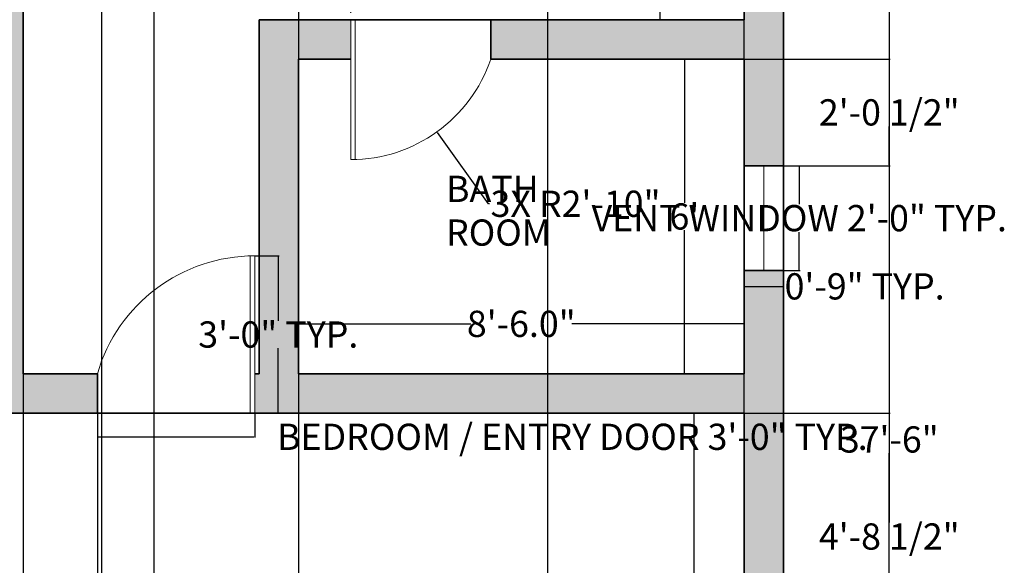
# Model space of a CAD drawing. Units: inches. Extents: x 1174 to 1615, y 3112 to 3628.
# Tile 5 of 6: x 1390 to 1615, y 3341 to 3466. Entities that reach past the tile are written whole.
import ezdxf

# ---------------------------------------------------------------- set-up
doc = ezdxf.new("R2010")
doc.units = ezdxf.units.IN
doc.header["$MEASUREMENT"] = 0
doc.layers.get('0').update_dxf_attribs({"color": 250})
for name, color, linetype, lineweight in [('A-ANNO-DIMS', 2, 'Continuous', 18), ('A-AREA-IDEN', 7, 'Continuous', 25), ('A-DOOR', 3, 'Continuous', 18), ('A-GLAZ', 4, 'Continuous', 18), ('A-WALL', 7, 'Continuous', 35)]:
    doc.layers.add(name, color=color, linetype=linetype, lineweight=lineweight)
doc.layers.add('A-WALL-PATT', color=18, linetype='Continuous', lineweight=13, true_color=0x000000)
doc.styles.get("Standard").update_dxf_attribs({"font": 'arial.ttf'})
doc.dimstyles.get("Standard").update_dxf_attribs({"dimtxt": 6, "dimasz": 0.18, "dimexe": 0.18, "dimexo": 0.0625, "dimgap": 0.09, "dimtad": 0, "dimtih": 1, "dimtoh": 1, "dimdec": 1, "dimzin": 0, "dimdsep": 46, "dimlunit": 3, "dimtxsty": 'Standard', "dimcen": 0.09, "dimadec": 0, "dimazin": 0, "dimtfac": 1, "dimtdec": 1, "dimtofl": 0, "dimtmove": 0, "dimatfit": 3, "dimfxl": 1, "dimtolj": 1, "dimtzin": 0, "dimarcsym": 0})

# ---------------------------------------------------------------- blocks, each defined once
blk = doc.blocks.new('*D9')
at = {"layer": 'A-ANNO-DIMS', "color": 0, "lineweight": -2, "transparency": 16777216}
for p, q in [((1453.66, 3385.09), (1453.66, 3396.65)), ((1453.84, 3396.47), (1493.1, 3396.47)), ((1555.48, 3396.47), (1516.23, 3396.47)), ((1555.66, 3385.09), (1555.66, 3396.65))]:
    blk.add_line(p, q, dxfattribs=at)
at = {"layer": 'A-ANNO-DIMS', "color": 0, "transparency": 16777216}
for points in [[(1453.84, 3396.5), (1453.84, 3396.44), (1453.66, 3396.47)], [(1555.48, 3396.5), (1555.48, 3396.44), (1555.66, 3396.47)]]:
    blk.add_solid(points, dxfattribs=at)
at = {"layer": 'Defpoints', "color": 0, "transparency": 16777216}
for p in [(1555.66, 3396.47), (1453.66, 3385.03), (1555.66, 3385.03)]:
    blk.add_point(p, dxfattribs=at)
at = {"layer": 'A-ANNO-DIMS', "color": 0, "transparency": 16777216, "insert": (1504.66, 3396.47), "char_height": 6, "attachment_point": 5}
blk.add_mtext('\\A1;8\'-6.0"', dxfattribs=at)
blk = doc.blocks.new('*D10')
at = {"layer": 'A-ANNO-DIMS', "color": 0, "lineweight": -2, "transparency": 16777216}
for p, q in [((1555.6, 3457.03), (1541.81, 3457.03)), ((1541.99, 3456.85), (1541.99, 3424.18)), ((1541.99, 3385.21), (1541.99, 3417.88)), ((1555.6, 3385.03), (1541.81, 3385.03))]:
    blk.add_line(p, q, dxfattribs=at)
at = {"layer": 'A-ANNO-DIMS', "color": 0, "transparency": 16777216}
for points in [[(1541.96, 3456.85), (1542.02, 3456.85), (1541.99, 3457.03)], [(1541.96, 3385.21), (1542.02, 3385.21), (1541.99, 3385.03)]]:
    blk.add_solid(points, dxfattribs=at)
at = {"layer": 'Defpoints', "color": 0, "transparency": 16777216}
for p in [(1555.66, 3457.03), (1541.99, 3385.03), (1555.66, 3385.03)]:
    blk.add_point(p, dxfattribs=at)
at = {"layer": 'A-ANNO-DIMS', "color": 0, "transparency": 16777216, "insert": (1541.99, 3421.03), "char_height": 6, "attachment_point": 5}
blk.add_mtext("\\A1;6'", dxfattribs=at)
blk = doc.blocks.new('*D12')
at = {"layer": 'A-ANNO-DIMS', "color": 0, "lineweight": -2, "transparency": 16777216}
for p, q in [((1555.6, 3376.03), (1544, 3376.03)), ((1544.18, 3375.85), (1544.18, 3283.18)), ((1544.18, 3184.21), (1544.18, 3276.88)), ((1555.6, 3184.03), (1544, 3184.03))]:
    blk.add_line(p, q, dxfattribs=at)
at = {"layer": 'A-ANNO-DIMS', "color": 0, "transparency": 16777216}
for points in [[(1544.15, 3375.85), (1544.21, 3375.85), (1544.18, 3376.03)], [(1544.15, 3184.21), (1544.21, 3184.21), (1544.18, 3184.03)]]:
    blk.add_solid(points, dxfattribs=at)
at = {"layer": 'Defpoints', "color": 0, "transparency": 16777216}
for p in [(1555.66, 3376.03), (1544.18, 3184.03), (1555.66, 3184.03)]:
    blk.add_point(p, dxfattribs=at)
at = {"layer": 'A-ANNO-DIMS', "color": 0, "transparency": 16777216, "insert": (1544.18, 3280.03), "char_height": 6, "attachment_point": 5}
blk.add_mtext("\\A1;16'", dxfattribs=at)
blk = doc.blocks.new('*D15')
at = {"layer": 'A-ANNO-DIMS', "color": 0, "lineweight": -2, "transparency": 16777216}
for p, q in [((1555.6, 3586.03), (1536.24, 3586.03)), ((1536.42, 3585.85), (1536.42, 3529.18)), ((1536.42, 3466.21), (1536.42, 3522.88)), ((1555.6, 3466.03), (1536.24, 3466.03))]:
    blk.add_line(p, q, dxfattribs=at)
at = {"layer": 'A-ANNO-DIMS', "color": 0, "transparency": 16777216}
for points in [[(1536.39, 3585.85), (1536.45, 3585.85), (1536.42, 3586.03)], [(1536.39, 3466.21), (1536.45, 3466.21), (1536.42, 3466.03)]]:
    blk.add_solid(points, dxfattribs=at)
at = {"layer": 'Defpoints', "color": 0, "transparency": 16777216}
for p in [(1555.66, 3586.03), (1536.42, 3466.03), (1555.66, 3466.03)]:
    blk.add_point(p, dxfattribs=at)
at = {"layer": 'A-ANNO-DIMS', "color": 0, "transparency": 16777216, "insert": (1536.42, 3526.03), "char_height": 6, "attachment_point": 5}
blk.add_mtext("\\A1;10'", dxfattribs=at)
blk = doc.blocks.new('DOOR-SWING-36IN')
for p, q in [((-1, 36), (-1, 0)), ((0, 0), (0, 36)), ((0, 0), (-36, 0))]:
    blk.add_line(p, q)
blk.add_arc((0, -1.5), 37.5, 90, 163.7398)
blk = doc.blocks.new('DOOR-SWING-32IN')
for p, q in [((0, 0), (0, -32)), ((0, 0), (32, 0)), ((1, -32), (1, 0))]:
    blk.add_line(p, q)
blk.add_arc((0, 1.76), 33.76, 270, 341.4134)
blk = doc.blocks.new('VENT-WINDOW-24IN')
for p, q in [((-4.5, -24), (-4.5, 0)), ((0, 0), (0, -24)), ((4.5, 0), (4.5, -24))]:
    blk.add_line(p, q)
blk = doc.blocks.new('*D28')
at = {"layer": 'A-ANNO-DIMS', "color": 0, "lineweight": -2, "transparency": 16777216}
for p, q in [((1564.73, 3432.64), (1568.44, 3432.64)), ((1568.26, 3432.46), (1568.26, 3423.83)), ((1568.26, 3408.82), (1568.26, 3417.44)), ((1564.73, 3408.64), (1568.44, 3408.64))]:
    blk.add_line(p, q, dxfattribs=at)
at = {"layer": 'A-ANNO-DIMS', "color": 0, "transparency": 16777216}
for points in [[(1568.23, 3432.46), (1568.29, 3432.46), (1568.26, 3432.64)], [(1568.23, 3408.82), (1568.29, 3408.82), (1568.26, 3408.64)]]:
    blk.add_solid(points, dxfattribs=at)
at = {"layer": 'Defpoints', "color": 0, "transparency": 16777216}
for p in [(1564.66, 3432.64), (1568.26, 3432.64), (1564.66, 3408.64)]:
    blk.add_point(p, dxfattribs=at)
at = {"layer": 'A-ANNO-DIMS', "color": 0, "transparency": 16777216, "insert": (1568.26, 3420.64), "char_height": 6, "attachment_point": 5}
blk.add_mtext('\\A1;VENT WINDOW 2\'-0" TYP.', dxfattribs=at)
blk = doc.blocks.new('*D29')
at = {"layer": 'A-ANNO-DIMS', "color": 0, "lineweight": -2, "transparency": 16777216}
for p, q in [((1555.66, 3408.58), (1555.66, 3404.86)), ((1564.66, 3408.58), (1564.66, 3404.86)), ((1555.84, 3405.04), (1564.48, 3405.04)), ((1564.66, 3405.04), (1564.84, 3405.04))]:
    blk.add_line(p, q, dxfattribs=at)
at = {"layer": 'A-ANNO-DIMS', "color": 0, "transparency": 16777216}
for points in [[(1555.84, 3405.07), (1555.84, 3405.01), (1555.66, 3405.04)], [(1564.48, 3405.07), (1564.48, 3405.01), (1564.66, 3405.04)]]:
    blk.add_solid(points, dxfattribs=at)
at = {"layer": 'Defpoints', "color": 0, "transparency": 16777216}
for p in [(1555.66, 3408.64), (1564.66, 3408.64), (1564.66, 3405.04)]:
    blk.add_point(p, dxfattribs=at)
at = {"layer": 'A-ANNO-DIMS', "color": 0, "transparency": 16777216, "insert": (1583.22, 3405.04), "char_height": 6, "attachment_point": 5}
blk.add_mtext('\\A1;0\'-9" TYP.', dxfattribs=at)
blk = doc.blocks.new('*D36')
at = {"layer": 'A-ANNO-DIMS', "color": 0, "lineweight": -2, "transparency": 16777216}
for p, q in [((1407.66, 3375.97), (1407.66, 3370.45)), ((1443.66, 3375.97), (1443.66, 3370.45)), ((1407.84, 3370.63), (1443.48, 3370.63)), ((1443.66, 3370.63), (1443.84, 3370.63))]:
    blk.add_line(p, q, dxfattribs=at)
at = {"layer": 'A-ANNO-DIMS', "color": 0, "transparency": 16777216}
for points in [[(1407.84, 3370.66), (1407.84, 3370.6), (1407.66, 3370.63)], [(1443.48, 3370.66), (1443.48, 3370.6), (1443.66, 3370.63)]]:
    blk.add_solid(points, dxfattribs=at)
at = {"layer": 'Defpoints', "color": 0, "transparency": 16777216}
for p in [(1407.66, 3376.03), (1443.66, 3376.03), (1443.66, 3370.63)]:
    blk.add_point(p, dxfattribs=at)
at = {"layer": 'A-ANNO-DIMS', "color": 0, "transparency": 16777216, "insert": (1516.34, 3370.63), "char_height": 6, "attachment_point": 5}
blk.add_mtext('\\A1;BEDROOM / ENTRY DOOR 3\'-0" TYP.', dxfattribs=at)
blk = doc.blocks.new('*D37')
at = {"layer": 'A-ANNO-DIMS', "color": 0, "lineweight": -2, "transparency": 16777216}
for p, q in [((1443.73, 3412.03), (1449.24, 3412.03)), ((1449.06, 3411.85), (1449.06, 3397.18)), ((1449.06, 3376.21), (1449.06, 3390.87)), ((1443.73, 3376.03), (1449.24, 3376.03))]:
    blk.add_line(p, q, dxfattribs=at)
at = {"layer": 'A-ANNO-DIMS', "color": 0, "transparency": 16777216}
for points in [[(1449.03, 3411.85), (1449.09, 3411.85), (1449.06, 3412.03)], [(1449.03, 3376.21), (1449.09, 3376.21), (1449.06, 3376.03)]]:
    blk.add_solid(points, dxfattribs=at)
at = {"layer": 'Defpoints', "color": 0, "transparency": 16777216}
for p in [(1443.66, 3412.03), (1449.06, 3412.03), (1443.66, 3376.03)]:
    blk.add_point(p, dxfattribs=at)
at = {"layer": 'A-ANNO-DIMS', "color": 0, "transparency": 16777216, "insert": (1449.06, 3394.03), "char_height": 6, "attachment_point": 5}
blk.add_mtext('\\A1;3\'-0" TYP.', dxfattribs=at)
blk = doc.blocks.new('*D41')
at = {"layer": 'A-ANNO-DIMS', "color": 0, "lineweight": -2, "transparency": 16777216}
for p, q in [((1564.73, 3595.03), (1589.04, 3595.03)), ((1588.86, 3594.85), (1588.86, 3373.18)), ((1588.86, 3145.21), (1588.86, 3366.87)), ((1439.51, 3145.03), (1589.04, 3145.03))]:
    blk.add_line(p, q, dxfattribs=at)
at = {"layer": 'A-ANNO-DIMS', "color": 0, "transparency": 16777216}
for points in [[(1588.83, 3594.85), (1588.89, 3594.85), (1588.86, 3595.03)], [(1588.83, 3145.21), (1588.89, 3145.21), (1588.86, 3145.03)]]:
    blk.add_solid(points, dxfattribs=at)
at = {"layer": 'Defpoints', "color": 0, "transparency": 16777216}
for p in [(1564.66, 3595.03), (1588.86, 3595.03), (1439.45, 3145.03)]:
    blk.add_point(p, dxfattribs=at)
at = {"layer": 'A-ANNO-DIMS', "color": 0, "transparency": 16777216, "insert": (1588.86, 3370.03), "char_height": 6, "attachment_point": 5}
blk.add_mtext('\\A1;37\'-6"', dxfattribs=at)
blk = doc.blocks.new('*D49')
at = {"layer": 'A-ANNO-DIMS', "color": 0, "lineweight": -2, "transparency": 16777216}
for p, q in [((1225.73, 3376.03), (1589.04, 3376.03)), ((1588.86, 3375.85), (1588.86, 3351.02)), ((1588.86, 3319.81), (1588.86, 3344.64)), ((1225.73, 3319.63), (1589.04, 3319.63))]:
    blk.add_line(p, q, dxfattribs=at)
at = {"layer": 'A-ANNO-DIMS', "color": 0, "transparency": 16777216}
for points in [[(1588.83, 3375.85), (1588.89, 3375.85), (1588.86, 3376.03)], [(1588.83, 3319.81), (1588.89, 3319.81), (1588.86, 3319.63)]]:
    blk.add_solid(points, dxfattribs=at)
at = {"layer": 'Defpoints', "color": 0, "transparency": 16777216}
for p in [(1225.66, 3376.03), (1225.66, 3319.63), (1588.86, 3319.63)]:
    blk.add_point(p, dxfattribs=at)
at = {"layer": 'A-ANNO-DIMS', "color": 0, "transparency": 16777216, "insert": (1588.86, 3347.83), "char_height": 6, "attachment_point": 5}
blk.add_mtext('\\A1;4\'-8 1/2"', dxfattribs=at)
blk = doc.blocks.new('*D51')
at = {"layer": 'A-ANNO-DIMS', "color": 0, "lineweight": -2, "transparency": 16777216}
for p, q in [((1555.73, 3457.03), (1589.04, 3457.03)), ((1588.86, 3456.85), (1588.86, 3448.03)), ((1588.86, 3432.82), (1588.86, 3441.64)), ((1564.73, 3432.64), (1589.04, 3432.64))]:
    blk.add_line(p, q, dxfattribs=at)
at = {"layer": 'A-ANNO-DIMS', "color": 0, "transparency": 16777216}
for points in [[(1588.83, 3456.85), (1588.89, 3456.85), (1588.86, 3457.03)], [(1588.83, 3432.82), (1588.89, 3432.82), (1588.86, 3432.64)]]:
    blk.add_solid(points, dxfattribs=at)
at = {"layer": 'Defpoints', "color": 0, "transparency": 16777216}
for p in [(1555.66, 3457.03), (1588.86, 3457.03), (1564.66, 3432.64)]:
    blk.add_point(p, dxfattribs=at)
at = {"layer": 'A-ANNO-DIMS', "color": 0, "transparency": 16777216, "insert": (1588.86, 3444.83), "char_height": 6, "attachment_point": 5}
blk.add_mtext('\\A1;2\'-0 1/2"', dxfattribs=at)
blk = doc.blocks.new('*D52')
at = {"layer": 'A-ANNO-DIMS', "color": 0, "lineweight": -2, "transparency": 16777216}
for p, q in [((1555.6, 3376.03), (1192.28, 3376.03)), ((1192.46, 3375.85), (1192.46, 3351.26)), ((1192.46, 3320.35), (1192.46, 3344.95)), ((1555.6, 3320.17), (1192.28, 3320.17))]:
    blk.add_line(p, q, dxfattribs=at)
at = {"layer": 'A-ANNO-DIMS', "color": 0, "transparency": 16777216}
for points in [[(1192.43, 3375.85), (1192.49, 3375.85), (1192.46, 3376.03)], [(1192.43, 3320.35), (1192.49, 3320.35), (1192.46, 3320.17)]]:
    blk.add_solid(points, dxfattribs=at)
at = {"layer": 'Defpoints', "color": 0, "transparency": 16777216}
for p in [(1555.66, 3376.03), (1192.46, 3320.17), (1555.66, 3320.17)]:
    blk.add_point(p, dxfattribs=at)
at = {"layer": 'A-ANNO-DIMS', "color": 0, "transparency": 16777216, "insert": (1192.46, 3348.1), "char_height": 6, "attachment_point": 5}
blk.add_mtext('\\A1;4\'-8"', dxfattribs=at)
blk = doc.blocks.new('*D57')
at = {"layer": 'A-ANNO-DIMS', "color": 0, "lineweight": -2, "transparency": 16777216}
for p, q in [((1390.66, 3384.97), (1390.66, 3120.65)), ((1407.66, 3384.97), (1407.66, 3120.65)), ((1390.84, 3120.83), (1391.38, 3120.83)), ((1407.48, 3120.83), (1406.95, 3120.83))]:
    blk.add_line(p, q, dxfattribs=at)
at = {"layer": 'A-ANNO-DIMS', "color": 0, "transparency": 16777216}
for points in [[(1390.84, 3120.86), (1390.84, 3120.8), (1390.66, 3120.83)], [(1407.48, 3120.86), (1407.48, 3120.8), (1407.66, 3120.83)]]:
    blk.add_solid(points, dxfattribs=at)
at = {"layer": 'Defpoints', "color": 0, "transparency": 16777216}
for p in [(1390.66, 3385.03), (1407.66, 3385.03), (1407.66, 3120.83)]:
    blk.add_point(p, dxfattribs=at)
at = {"layer": 'A-ANNO-DIMS', "color": 0, "transparency": 16777216, "insert": (1399.16, 3120.83), "char_height": 6, "attachment_point": 5}
blk.add_mtext('\\A1;1\'-5"', dxfattribs=at)
blk = doc.blocks.new('*D59')
at = {"layer": 'A-ANNO-DIMS', "color": 0, "lineweight": -2, "transparency": 16777216}
for p, q in [((1408.66, 3268.09), (1408.66, 3619.41)), ((1408.84, 3619.23), (1420.48, 3619.23)), ((1420.66, 3268.09), (1420.66, 3619.41)), ((1420.66, 3619.23), (1420.84, 3619.23))]:
    blk.add_line(p, q, dxfattribs=at)
at = {"layer": 'A-ANNO-DIMS', "color": 0, "transparency": 16777216}
for points in [[(1408.84, 3619.26), (1408.84, 3619.2), (1408.66, 3619.23)], [(1420.48, 3619.26), (1420.48, 3619.2), (1420.66, 3619.23)]]:
    blk.add_solid(points, dxfattribs=at)
at = {"layer": 'Defpoints', "color": 0, "transparency": 16777216}
for p in [(1420.66, 3619.23), (1408.66, 3268.03), (1420.66, 3268.03)]:
    blk.add_point(p, dxfattribs=at)
at = {"layer": 'A-ANNO-DIMS', "color": 0, "transparency": 16777216, "insert": (1428.63, 3619.23), "char_height": 6, "attachment_point": 5}
blk.add_mtext('\\A1;1\'-0"', dxfattribs=at)
blk = doc.blocks.new('*D70')
at = {"layer": 'A-ANNO-DIMS', "color": 0, "lineweight": -2, "transparency": 16777216}
for p, q in [((1390.66, 3585.97), (1390.66, 3120.65)), ((1453.68, 3583.03), (1453.68, 3120.65)), ((1390.84, 3120.83), (1414.11, 3120.83)), ((1453.5, 3120.83), (1430.24, 3120.83))]:
    blk.add_line(p, q, dxfattribs=at)
at = {"layer": 'A-ANNO-DIMS', "color": 0, "transparency": 16777216}
for points in [[(1390.84, 3120.86), (1390.84, 3120.8), (1390.66, 3120.83)], [(1453.5, 3120.86), (1453.5, 3120.8), (1453.68, 3120.83)]]:
    blk.add_solid(points, dxfattribs=at)
at = {"layer": 'Defpoints', "color": 0, "transparency": 16777216}
for p in [(1390.66, 3586.03), (1453.68, 3583.1), (1453.68, 3120.83)]:
    blk.add_point(p, dxfattribs=at)
at = {"layer": 'A-ANNO-DIMS', "color": 0, "transparency": 16777216, "insert": (1422.17, 3120.83), "char_height": 6, "attachment_point": 5}
blk.add_mtext('\\A1;5\'-3"', dxfattribs=at)
blk = doc.blocks.new('*D73')
at = {"layer": 'A-ANNO-DIMS', "color": 0, "lineweight": -2, "transparency": 16777216}
for p, q in [((1510.72, 3286.5), (1510.72, 3619.41)), ((1510.9, 3619.23), (1525.13, 3619.23)), ((1555.48, 3619.23), (1541.25, 3619.23)), ((1555.66, 3284.24), (1555.66, 3619.41))]:
    blk.add_line(p, q, dxfattribs=at)
at = {"layer": 'A-ANNO-DIMS', "color": 0, "transparency": 16777216}
for points in [[(1510.9, 3619.26), (1510.9, 3619.2), (1510.72, 3619.23)], [(1555.48, 3619.26), (1555.48, 3619.2), (1555.66, 3619.23)]]:
    blk.add_solid(points, dxfattribs=at)
at = {"layer": 'Defpoints', "color": 0, "transparency": 16777216}
for p in [(1510.72, 3619.23), (1510.72, 3286.44), (1555.66, 3284.17)]:
    blk.add_point(p, dxfattribs=at)
at = {"layer": 'A-ANNO-DIMS', "color": 0, "transparency": 16777216, "insert": (1533.19, 3619.23), "char_height": 6, "attachment_point": 5}
blk.add_mtext('\\A1;3\'-9"', dxfattribs=at)
blk = doc.blocks.new('*D77')
at = {"layer": 'A-ANNO-DIMS', "color": 0, "lineweight": -2, "transparency": 16777216}
for p, q in [((1465.57, 3467.79), (1465.75, 3467.79)), ((1465.66, 3467.7), (1465.66, 3467.88)), ((1497.19, 3423.93), (1485.47, 3440.23)), ((1497.37, 3423.93), (1497.19, 3423.93))]:
    blk.add_line(p, q, dxfattribs=at)
at = {"layer": 'A-ANNO-DIMS', "color": 0, "transparency": 16777216}
blk.add_solid([(1485.5, 3440.25), (1485.45, 3440.21), (1485.37, 3440.38)], dxfattribs=at)
at = {"layer": 'Defpoints', "color": 0, "transparency": 16777216}
for p in [(1465.66, 3467.79), (1485.37, 3440.38)]:
    blk.add_point(p, dxfattribs=at)
at = {"layer": 'A-ANNO-DIMS', "color": 0, "transparency": 16777216, "insert": (1517.08, 3423.93), "char_height": 6, "attachment_point": 5}
blk.add_mtext('\\A1;3X R2\'-10"', dxfattribs=at)

msp = doc.modelspace()

# ---------------------------------------------------------------- hatches: boundary and pattern name
at = {"layer": 'A-WALL-PATT'}
h = msp.add_hatch(color=256, dxfattribs=at)
h.dxf.hatch_style = 1
h.paths.add_polyline_path([(1564.66, 3595.03), (1216.66, 3595.03), (1216.66, 3564.55), (1225.66, 3564.55), (1225.66, 3586.03), (1381.66, 3586.03), (1381.66, 3385.03), (1380.66, 3385.03), (1380.66, 3376.03), (1381.66, 3376.03), (1407.66, 3376.03), (1407.66, 3385.03), (1390.66, 3385.03), (1390.66, 3586.03), (1555.66, 3586.03), (1555.66, 3558.83), (1564.66, 3558.83)])
h.paths.add_polyline_path([(1564.66, 3408.64), (1555.66, 3408.64), (1555.66, 3385.03), (1453.66, 3385.03), (1453.66, 3457.03), (1465.66, 3457.03), (1465.66, 3466.03), (1453.66, 3466.03), (1444.66, 3466.03), (1444.66, 3385.03), (1443.66, 3385.03), (1443.66, 3376.03), (1444.66, 3376.03), (1555.66, 3376.03), (1555.66, 3320.17), (1564.66, 3320.17)])
h.paths.add_polyline_path([(1564.66, 3522.83), (1555.66, 3522.83), (1555.66, 3466.03), (1497.66, 3466.03), (1497.66, 3457.03), (1555.66, 3457.03), (1555.66, 3432.64), (1564.66, 3432.64)], flags=17)
h.paths.add_polyline_path([(1344.66, 3385.03), (1336.66, 3385.03), (1336.66, 3466.03), (1269.66, 3466.03), (1269.66, 3457.03), (1327.66, 3457.03), (1327.66, 3385.03), (1225.66, 3385.03), (1225.66, 3413.31), (1216.66, 3413.31), (1216.66, 3319.63), (1225.66, 3319.63), (1225.66, 3376.03), (1344.66, 3376.03)])
h.paths.add_polyline_path([(1237.66, 3466.03), (1225.66, 3466.03), (1225.66, 3528.55), (1216.66, 3528.55), (1216.66, 3437.31), (1225.66, 3437.31), (1225.66, 3457.03), (1237.66, 3457.03)], flags=17)
h.paths.add_polyline_path([(1265.25, 3184.03), (1225.66, 3184.03), (1225.66, 3283.63), (1216.66, 3283.63), (1216.66, 3175.03), (1265.25, 3175.03)])
h.paths.add_polyline_path([(1372.66, 3184.03), (1360.66, 3184.03), (1360.66, 3268.03), (1376.66, 3268.03), (1376.66, 3277.03), (1360.66, 3277.03), (1360.66, 3313.03), (1351.66, 3313.03), (1351.66, 3184.03), (1301.25, 3184.03), (1301.25, 3175.03), (1372.66, 3175.03)])
h.paths.add_polyline_path([(1460.02, 3184.03), (1429.66, 3184.03), (1429.66, 3277.03), (1408.66, 3277.03), (1408.66, 3268.03), (1420.66, 3268.03), (1420.66, 3184.03), (1408.66, 3184.03), (1408.66, 3175.03), (1460.02, 3175.03)])
h.paths.add_polyline_path([(1564.66, 3284.17), (1555.66, 3284.17), (1555.66, 3184.03), (1520.02, 3184.03), (1520.02, 3175.03), (1564.66, 3175.03)])

# ---------------------------------------------------------------- linework, layer by layer
at = {"layer": 'A-DOOR'}
for p, q in [((1465.66, 3434.03), (1465.66, 3466.03)), ((1443.66, 3412.03), (1443.66, 3376.03))]:
    msp.add_line(p, q, dxfattribs=at)
at = {"layer": 'A-WALL'}
for p, q in [((1564.66, 3595.03), (1564.66, 3175.03)), ((1390.66, 3586.03), (1390.66, 3385.03)), ((1555.66, 3586.03), (1555.66, 3466.03)), ((1444.66, 3466.03), (1444.66, 3385.03)), ((1444.66, 3466.03), (1555.66, 3466.03)), ((1453.66, 3466.03), (1465.66, 3466.03)), ((1497.66, 3466.03), (1497.66, 3457.03)), ((1453.66, 3457.03), (1453.66, 3385.03)), ((1453.66, 3457.03), (1465.66, 3457.03)), ((1497.66, 3457.03), (1555.66, 3457.03)), ((1555.66, 3457.03), (1555.66, 3385.03)), ((1555.66, 3432.64), (1564.66, 3432.64)), ((1564.66, 3408.64), (1555.66, 3408.64)), ((1390.66, 3385.03), (1407.66, 3385.03)), ((1407.66, 3376.03), (1407.66, 3385.03)), ((1443.66, 3385.03), (1444.66, 3385.03)), ((1453.66, 3385.03), (1555.66, 3385.03)), ((1225.66, 3376.03), (1555.66, 3376.03)), ((1444.66, 3376.03), (1443.66, 3376.03)), ((1555.66, 3376.03), (1555.66, 3184.03))]:
    msp.add_line(p, q, dxfattribs=at)

# ---------------------------------------------------------------- block references
at = {"layer": 'A-DOOR'}
for name, p in [('DOOR-SWING-32IN', (1465.66, 3466.03)), ('DOOR-SWING-36IN', (1443.66, 3376.03))]:
    msp.add_blockref(name, p, dxfattribs=at)
at = {"layer": 'A-GLAZ'}
msp.add_blockref('VENT-WINDOW-24IN', (1560.16, 3432.64), dxfattribs=at)

# ---------------------------------------------------------------- texts
at = {"layer": 'A-AREA-IDEN', "insert": (1487.44, 3430.34), "char_height": 6, "attachment_point": 1}
msp.add_mtext_dynamic_manual_height_columns('BATH\\PROOM', width=57.8599, gutter_width=1, heights=[0], dxfattribs=at)

# ---------------------------------------------------------------- dimensions: what is measured, and where the dimension line sits
at = {"layer": 'A-ANNO-DIMS'}
for base, p1, p2, override, picture, middle in [((1420.66, 3619.23), (1408.66, 3268.03), (1420.66, 3268.03), {"dimdec": 1, "dimlfac": 1, "dimrnd": 0, "dimzin": 1, "dimdsep": 46, "dimlunit": 4, "dimfrac": 2}, '*D59', (1428.63, 3619.23)), ((1510.72, 3619.23), (1555.66, 3284.17), (1510.72, 3286.44), {"dimdec": 1, "dimlfac": 1, "dimrnd": 0, "dimzin": 1, "dimdsep": 46, "dimlunit": 4, "dimfrac": 2}, '*D73', (1533.19, 3619.23)), ((1453.68, 3120.83), (1390.66, 3586.03), (1453.68, 3583.1), {"dimdec": 1, "dimlfac": 1, "dimrnd": 0, "dimzin": 1, "dimdsep": 46, "dimlunit": 4, "dimfrac": 2}, '*D70', (1422.17, 3120.83)), ((1555.66, 3396.47), (1453.66, 3385.03), (1555.66, 3385.03), {"dimclrd": 0, "dimclre": 0, "dimclrt": 0}, '*D9', (1504.66, 3396.47)), ((1407.66, 3120.83), (1390.66, 3385.03), (1407.66, 3385.03), {"dimdec": 1, "dimlfac": 1, "dimrnd": 0, "dimzin": 1, "dimdsep": 46, "dimlunit": 4, "dimfrac": 2}, '*D57', (1399.16, 3120.83))]:
    dim = msp.add_linear_dim(base=base, p1=p1, p2=p2, dimstyle='Standard', override=override, dxfattribs=at)
    dim.commit()
    dim.dimension.update_dxf_attribs({"geometry": picture, "text_midpoint": middle})
for base, p1, p2, override, picture, middle in [((1588.86, 3595.03), (1439.45, 3145.03), (1564.66, 3595.03), {"dimdec": 1, "dimlfac": 1, "dimrnd": 0, "dimzin": 1, "dimdsep": 46, "dimlunit": 4, "dimfrac": 2}, '*D41', (1588.86, 3370.03)), ((1536.42, 3466.03), (1555.66, 3586.03), (1555.66, 3466.03), {"dimclrd": 0, "dimclre": 0, "dimclrt": 0}, '*D15', (1536.42, 3526.03)), ((1541.99, 3385.03), (1555.66, 3457.03), (1555.66, 3385.03), {"dimclrd": 0, "dimclre": 0, "dimclrt": 0}, '*D10', (1541.99, 3421.03)), ((1588.86, 3457.03), (1564.66, 3432.64), (1555.66, 3457.03), {"dimdec": 1, "dimlfac": 1, "dimrnd": 0, "dimzin": 1, "dimdsep": 46, "dimlunit": 4, "dimfrac": 2}, '*D51', (1588.86, 3444.83)), ((1192.46, 3320.17), (1555.66, 3376.03), (1555.66, 3320.17), {"dimdec": 1, "dimlfac": 1, "dimrnd": 0, "dimzin": 1, "dimdsep": 46, "dimlunit": 4, "dimfrac": 2}, '*D52', (1192.46, 3348.1)), ((1588.86, 3319.63), (1225.66, 3376.03), (1225.66, 3319.63), {"dimdec": 1, "dimlfac": 1, "dimrnd": 0, "dimzin": 1, "dimdsep": 46, "dimlunit": 4, "dimfrac": 2}, '*D49', (1588.86, 3347.83)), ((1544.18, 3184.03), (1555.66, 3376.03), (1555.66, 3184.03), {"dimclrd": 0, "dimclre": 0, "dimclrt": 0}, '*D12', (1544.18, 3280.03))]:
    dim = msp.add_linear_dim(base=base, p1=p1, p2=p2, angle=90, dimstyle='Standard', override=override, dxfattribs=at)
    dim.commit()
    dim.dimension.update_dxf_attribs({"geometry": picture, "text_midpoint": middle})
dim = msp.add_radius_dim(center=(1465.66, 3467.79), mpoint=(1485.37, 3440.38), text='3X <>', dimstyle='Standard', override={"dimdec": 1, "dimlfac": 1, "dimrnd": 0, "dimzin": 1, "dimdsep": 46, "dimlunit": 4, "dimfrac": 2}, dxfattribs=at)
dim.commit()
dim.dimension.update_dxf_attribs({"geometry": '*D77', "text_midpoint": (1517.08, 3423.93), "dimtype": 164})
for base, p1, p2, text, picture, middle in [((1568.26, 3432.64), (1564.66, 3408.64), (1564.66, 3432.64), 'VENT WINDOW <> TYP.', '*D28', (1568.26, 3420.64)), ((1449.06, 3412.03), (1443.66, 3376.03), (1443.66, 3412.03), '<> TYP.', '*D37', (1449.06, 3394.03))]:
    dim = msp.add_linear_dim(base=base, p1=p1, p2=p2, angle=90, text=text, dimstyle='Standard', override={"dimdec": 1, "dimlfac": 1, "dimrnd": 0, "dimzin": 1, "dimdsep": 46, "dimlunit": 4, "dimfrac": 2}, dxfattribs=at)
    dim.commit()
    dim.dimension.update_dxf_attribs({"geometry": picture, "text_midpoint": middle})
for base, p1, p2, text, picture, middle in [((1564.66, 3405.04), (1555.66, 3408.64), (1564.66, 3408.64), '<> TYP.', '*D29', (1583.22, 3405.04)), ((1443.66, 3370.63), (1407.66, 3376.03), (1443.66, 3376.03), 'BEDROOM / ENTRY DOOR <> TYP.', '*D36', (1516.34, 3370.63))]:
    dim = msp.add_linear_dim(base=base, p1=p1, p2=p2, text=text, dimstyle='Standard', override={"dimdec": 1, "dimlfac": 1, "dimrnd": 0, "dimzin": 1, "dimdsep": 46, "dimlunit": 4, "dimfrac": 2}, dxfattribs=at)
    dim.commit()
    dim.dimension.update_dxf_attribs({"geometry": picture, "text_midpoint": middle})

doc.saveas('drawing.dxf')
